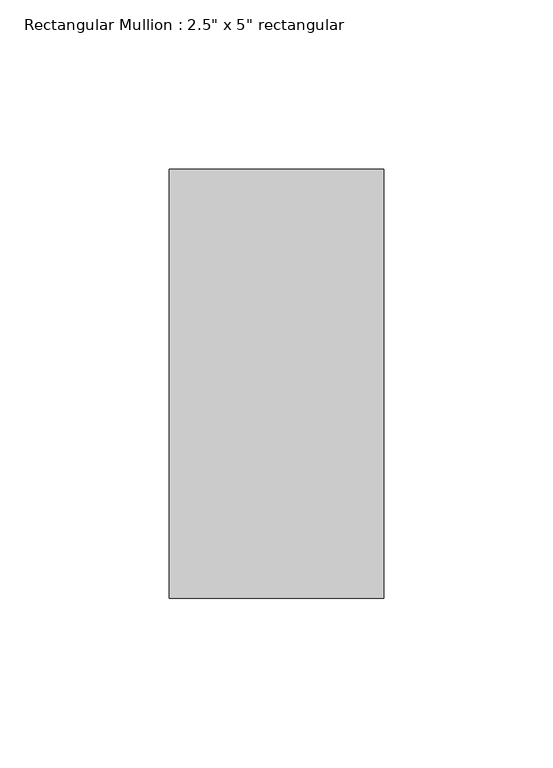
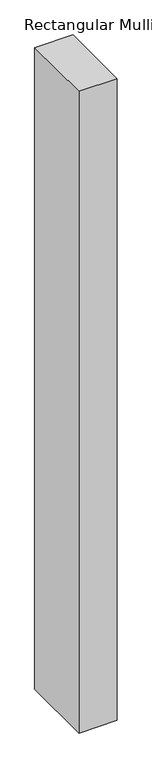
"""IFC4 building model written with IfcOpenShell, lengths in millimetres: member geometry."""

from ifc_helpers import new_model, si_unit, frame, origin, place, context, project, spatial, polyline, outline, extrude, source, transform, mapped, element, save


def member_cd6cc0cf(model_context):
    return source(origin(), model_context, "Body", "SweptSolid", [
        extrude(outline(polyline([(0.0, 63.5), (0.0, -63.5), (-63.5, -63.5), (-63.5, 63.5), (0.0, 63.5)])), frame((0.0, 0.0, -1125.4924454), z_axis=(0.0, 0.0, 1.0), x_axis=(1.0, 0.0, 0.0)), (0.0, 0.0, 1.0), 1125.4924454),
    ])


if __name__ == "__main__":
    model = new_model("IFC4")
    model_context = context("Model", 3, world=origin())
    ifc_project = project(units=[si_unit("LENGTHUNIT", "METRE", prefix="MILLI")], contexts=[model_context])
    site = spatial("IfcSite", under=ifc_project)
    building = spatial("IfcBuilding", under=site)
    placement = place(None, origin())
    member_shape = member_cd6cc0cf(model_context)
    element("IfcMember", 1, ObjectType="Rectangular Mullion : 2.5\" x 5\" rectangular", at=placement, inside=building, context=model_context, shape_type="MappedRepresentation", body=[
        mapped(member_shape, transform((0.0, 0.0, 0.0), x_axis=(1.0, 0.0, 0.0), y_axis=(0.0, 1.0, 0.0), z_axis=(0.0, 0.0, 1.0))),
    ])
    save(model, "model.ifc")

# Revit data of these elements
# Type "Rectangular Mullion : 2.5\" x 5\" rectangular"
#   built-in parameter 1007304 = 0.416667 (stored number, unit not read)
#   built-in parameter 1007301 = 0.104167 (stored number, unit not read)
#   built-in parameter 1007300 = 0.104167 (stored number, unit not read)
# Element 1 (IfcMember, "Rectangular Mullion : 2.5\" x 5\" rectangular")
#   Materials on its faces: "BLACK COLOUR"
# Materials
#   "BLACK COLOUR": class "Generic", colour RGB 120 120 120, transparency 0, Cost = 0
